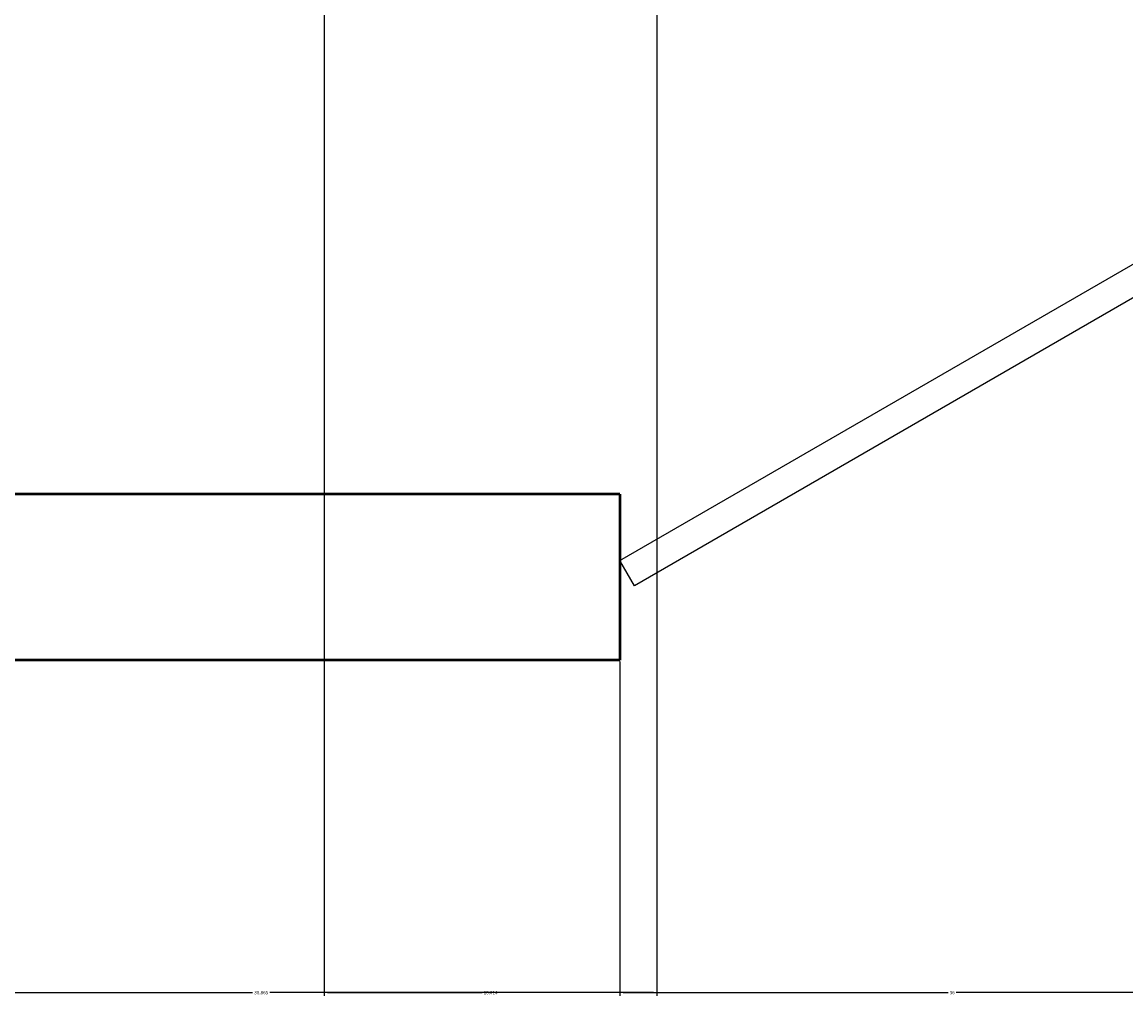
# Model space of a CAD drawing. Units: inches. Extents: x 2621 to 2849, y 2066 to 2463.
# Tile 3 of 28: x 2729 to 2789, y 2066 to 2119. Entities that reach past the tile are written whole.
import ezdxf

# ---------------------------------------------------------------- set-up
doc = ezdxf.new("R2010")
doc.units = ezdxf.units.IN
for name, color, linetype, lineweight in [('A-ANNO-DIMS', 2, 'Continuous', 18), ('A-DOOR', 3, 'Continuous', 25), ('A-WALL', 7, 'Continuous', 50)]:
    doc.layers.add(name, color=color, linetype=linetype, lineweight=lineweight)
doc.styles.get("Standard").update_dxf_attribs({"font": 'arial.ttf'})
doc.dimstyles.get("Standard").update_dxf_attribs({"dimtxt": 0.18, "dimasz": 0.18, "dimexe": 0.18, "dimexo": 0.0625, "dimgap": 0.09, "dimtad": 0, "dimtih": 1, "dimtoh": 1, "dimdec": 4, "dimzin": 0, "dimdsep": 46, "dimtxsty": 'Standard', "dimcen": 0.09, "dimadec": 0, "dimazin": 0, "dimtfac": 1, "dimtdec": 4, "dimtofl": 0, "dimtmove": 0, "dimatfit": 3, "dimfxl": 1, "dimtolj": 1, "dimtzin": 0, "dimarcsym": 0})

# ---------------------------------------------------------------- blocks, each defined once
blk = doc.blocks.new('*U4')
for p, q in [((0, 0), (0, -6)), ((40, 0), (40, -6))]:
    blk.add_line(p, q)
blk.add_lwpolyline([(0, 0), (34.641, 20), (35.516, 18.484), (0.875, -1.516)], close=True)
blk.add_arc((0, 0), 40, 0, 30)
blk = doc.blocks.new('*D41')
at = {"layer": 'A-ANNO-DIMS', "color": 0, "lineweight": -2, "transparency": 16777216}
for p, q in [((2723.005, 2084.312), (2723.005, 2066.191)), ((2761.87, 2084.312), (2761.87, 2066.191)), ((2723.185, 2066.371), (2741.973, 2066.371)), ((2761.69, 2066.371), (2742.902, 2066.371))]:
    blk.add_line(p, q, dxfattribs=at)
at = {"layer": 'A-ANNO-DIMS', "color": 0, "transparency": 16777216}
for points in [[(2723.185, 2066.401), (2723.185, 2066.341), (2723.005, 2066.371)], [(2761.69, 2066.401), (2761.69, 2066.341), (2761.87, 2066.371)]]:
    blk.add_solid(points, dxfattribs=at)
at = {"layer": 'Defpoints', "color": 0, "transparency": 16777216}
for p in [(2723.005, 2084.375), (2761.87, 2084.375), (2761.87, 2066.371)]:
    blk.add_point(p, dxfattribs=at)
at = {"layer": 'A-ANNO-DIMS', "color": 0, "transparency": 16777216, "insert": (2742.437, 2066.371), "char_height": 0.18, "attachment_point": 5}
blk.add_mtext('\\A1;38.865', dxfattribs=at)
blk = doc.blocks.new('*D42')
at = {"layer": 'A-ANNO-DIMS', "color": 0, "lineweight": -2, "transparency": 16777216}
for p, q in [((2761.87, 2084.312), (2761.87, 2066.191)), ((2797.87, 2084.312), (2797.87, 2066.191)), ((2762.05, 2066.371), (2779.651, 2066.371)), ((2797.69, 2066.371), (2780.089, 2066.371))]:
    blk.add_line(p, q, dxfattribs=at)
at = {"layer": 'A-ANNO-DIMS', "color": 0, "transparency": 16777216}
for points in [[(2762.05, 2066.401), (2762.05, 2066.341), (2761.87, 2066.371)], [(2797.69, 2066.401), (2797.69, 2066.341), (2797.87, 2066.371)]]:
    blk.add_solid(points, dxfattribs=at)
at = {"layer": 'Defpoints', "color": 0, "transparency": 16777216}
for p in [(2761.87, 2084.375), (2797.87, 2084.375), (2797.87, 2066.371)]:
    blk.add_point(p, dxfattribs=at)
at = {"layer": 'A-ANNO-DIMS', "color": 0, "transparency": 16777216, "insert": (2779.87, 2066.371), "char_height": 0.18, "attachment_point": 5}
blk.add_mtext('\\A1;36', dxfattribs=at)
blk = doc.blocks.new('*D70')
at = {"layer": 'A-ANNO-DIMS', "color": 0, "lineweight": -2, "transparency": 16777216}
for p, q in [((2745.856, 2291.312), (2745.856, 2066.191)), ((2763.87, 2291.312), (2763.87, 2066.191)), ((2746.036, 2066.371), (2754.408, 2066.371)), ((2763.69, 2066.371), (2755.318, 2066.371))]:
    blk.add_line(p, q, dxfattribs=at)
at = {"layer": 'A-ANNO-DIMS', "color": 0, "transparency": 16777216}
for points in [[(2746.036, 2066.401), (2746.036, 2066.341), (2745.856, 2066.371)], [(2763.69, 2066.401), (2763.69, 2066.341), (2763.87, 2066.371)]]:
    blk.add_solid(points, dxfattribs=at)
at = {"layer": 'Defpoints', "color": 0, "transparency": 16777216}
for p in [(2745.856, 2291.375), (2763.87, 2291.375), (2763.87, 2066.371)]:
    blk.add_point(p, dxfattribs=at)
at = {"layer": 'A-ANNO-DIMS', "color": 0, "transparency": 16777216, "insert": (2754.863, 2066.371), "char_height": 0.18, "attachment_point": 5}
blk.add_mtext('\\A1;18.014', dxfattribs=at)

msp = doc.modelspace()

# ---------------------------------------------------------------- linework, layer by layer
at = {"layer": 'A-WALL'}
for q in [(2647.8701, 2093.3746), (2761.8701, 2084.3746)]:
    msp.add_line((2761.8701, 2093.3746), q, dxfattribs=at)
msp.add_lwpolyline([(2761.8701, 2084.3746), (2638.8701, 2084.3746), (2638.8701, 2444.3746), (2830.8701, 2444.3746), (2830.8701, 2084.3746), (2797.8701, 2084.3746)], dxfattribs=at)

# ---------------------------------------------------------------- block references
at = {"layer": 'A-DOOR', "xscale": 0.9, "yscale": 0.9, "zscale": 0.9}
msp.add_blockref('*U4', (2761.8701, 2089.7746), dxfattribs=at)

# ---------------------------------------------------------------- dimensions: what is measured, and where the dimension line sits
at = {"layer": 'A-ANNO-DIMS'}
for base, p1, p2, override, picture, middle in [((2763.8701, 2066.3711), (2745.8562, 2291.3746), (2763.8701, 2291.3746), {"dimdec": 3, "dimlfac": 1, "dimrnd": 0, "dimzin": 0, "dimdsep": 46, "dimlunit": 2}, '*D70', (2754.8631, 2066.3711)), ((2761.8701, 2066.3711), (2723.0048, 2084.3746), (2761.8701, 2084.3746), {"dimdec": 3, "dimlfac": 1, "dimrnd": 0, "dimzin": 0, "dimdsep": 46, "dimlunit": 2}, '*D41', (2742.4374, 2066.3711)), ((2797.8701, 2066.3711), (2761.8701, 2084.3746), (2797.8701, 2084.3746), {"dimdec": 0, "dimlfac": 1, "dimrnd": 0, "dimzin": 0, "dimdsep": 46, "dimlunit": 2}, '*D42', (2779.8701, 2066.3711))]:
    dim = msp.add_linear_dim(base=base, p1=p1, p2=p2, dimstyle='Standard', override=override, dxfattribs=at)
    dim.commit()
    dim.dimension.update_dxf_attribs({"geometry": picture, "text_midpoint": middle})

doc.saveas('drawing.dxf')
